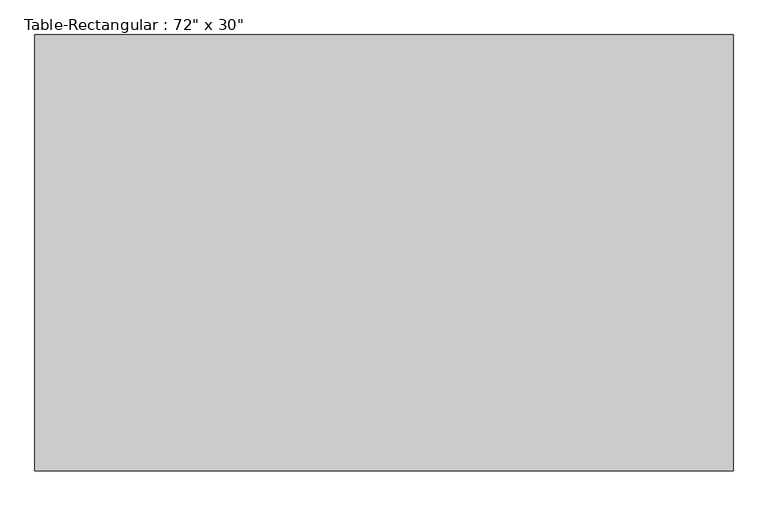
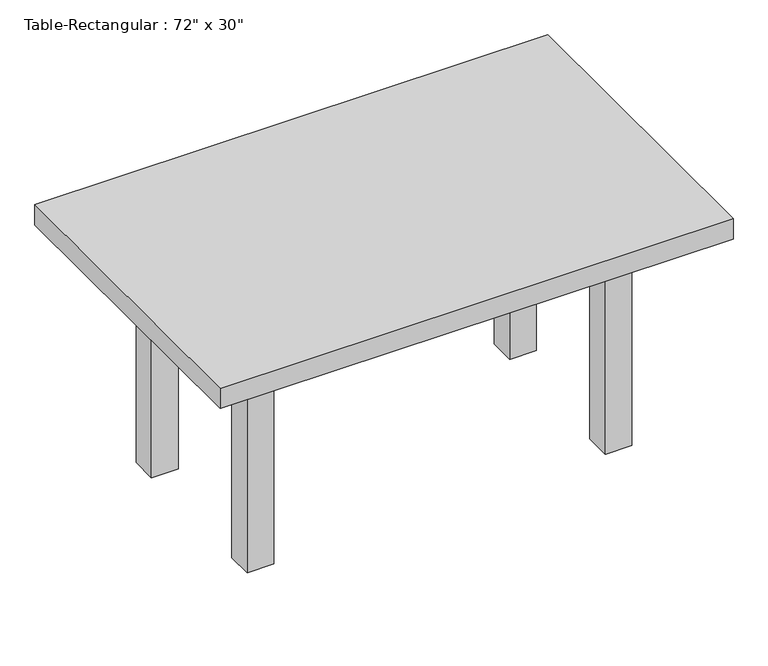
"""IFC4 building model written with IfcOpenShell, lengths in millimetres: furniture geometry."""

from ifc_helpers import new_model, si_unit, frame, origin, origin_with_axes, place, context, project, spatial, polyline, outline, extrude, source, transform, mapped, element, save


def furniture_1bba2e14(model_context):
    return source(origin(), model_context, "Body", "SweptSolid", [
        extrude(outline(polyline([(393.7, 190.5), (393.7, 165.1), (-393.7, 165.1), (-393.7, 190.5), (393.7, 190.5)])), frame((0.0, 0.0, 457.2), z_axis=(0.0, 0.0, 1.0), x_axis=(1.0, 0.0, 0.0)), (0.0, 0.0, 1.0), 101.6),
        extrude(outline(polyline([(393.7, -190.5), (-393.7, -190.5), (-393.7, -165.1), (393.7, -165.1), (393.7, -190.5)])), frame((0.0, 0.0, 457.2), z_axis=(0.0, 0.0, 1.0), x_axis=(1.0, 0.0, 0.0)), (0.0, 0.0, 1.0), 101.6),
        extrude(outline(polyline([(-406.4, -165.1), (-431.8, -165.1), (-431.8, 165.1), (-406.4, 165.1), (-406.4, -165.1)])), frame((0.0, 0.0, 457.2), z_axis=(0.0, 0.0, 1.0), x_axis=(1.0, 0.0, 0.0)), (0.0, 0.0, 1.0), 101.6),
        extrude(outline(polyline([(406.4, -165.1), (406.4, 165.1), (431.8, 165.1), (431.8, -165.1), (406.4, -165.1)])), frame((0.0, 0.0, 457.2), z_axis=(0.0, 0.0, 1.0), x_axis=(1.0, 0.0, 0.0)), (0.0, 0.0, 1.0), 101.6),
        extrude(outline(polyline([(609.6, 381.0), (609.6, -381.0), (-609.6, -381.0), (-609.6, 381.0), (609.6, 381.0)])), frame((0.0, 0.0, 558.8), z_axis=(0.0, 0.0, 1.0), x_axis=(1.0, 0.0, 0.0)), (0.0, 0.0, 1.0), 50.8),
        extrude(outline(polyline([(-393.7, 228.6), (-393.7, 165.1), (-457.2, 165.1), (-457.2, 228.6), (-393.7, 228.6)])), origin_with_axes(), (0.0, 0.0, 1.0), 558.8),
        extrude(outline(polyline([(393.7, 228.6), (457.2, 228.6), (457.2, 165.1), (393.7, 165.1), (393.7, 228.6)])), origin_with_axes(), (0.0, 0.0, 1.0), 558.8),
        extrude(outline(polyline([(-393.7, -228.6), (-457.2, -228.6), (-457.2, -165.1), (-393.7, -165.1), (-393.7, -228.6)])), origin_with_axes(), (0.0, 0.0, 1.0), 558.8),
        extrude(outline(polyline([(393.7, -228.6), (393.7, -165.1), (457.2, -165.1), (457.2, -228.6), (393.7, -228.6)])), origin_with_axes(), (0.0, 0.0, 1.0), 558.8),
    ])


if __name__ == "__main__":
    model = new_model("IFC4")
    model_context = context("Model", 3, world=origin())
    ifc_project = project(units=[si_unit("LENGTHUNIT", "METRE", prefix="MILLI")], contexts=[model_context])
    site = spatial("IfcSite", under=ifc_project)
    building = spatial("IfcBuilding", under=site)
    placement = place(None, origin())
    furniture_shape = furniture_1bba2e14(model_context)
    element("IfcFurniture", 1, ObjectType="Table-Rectangular : 72\" x 30\"", at=placement, inside=building, context=model_context, shape_type="MappedRepresentation", body=[
        mapped(furniture_shape, transform((0.0, 0.0, 0.0), x_axis=(1.0, 0.0, 0.0), y_axis=(0.0, 1.0, 0.0), z_axis=(0.0, 0.0, 1.0))),
    ])
    save(model, "model.ifc")

# Revit data of these elements
# Type "Table-Rectangular : 72\" x 30\""
#   Assembly Code = "E2020200"
#   Height = 2' - 0"
#   Length = 4' - 0"
#   Width = 2' - 6"
#   Base Material = Birch
#   Top Material = Birch
#   Default Elevation = 0
# Element 1 (IfcFurniture, "Table-Rectangular : 72\" x 30\"")
#   Materials on its faces: "Birch"
# Materials
#   "Birch": class "Wood", colour RGB 224 178 126, transparency 0, Description = "Betula Alleghaniensis", Cost = 0
